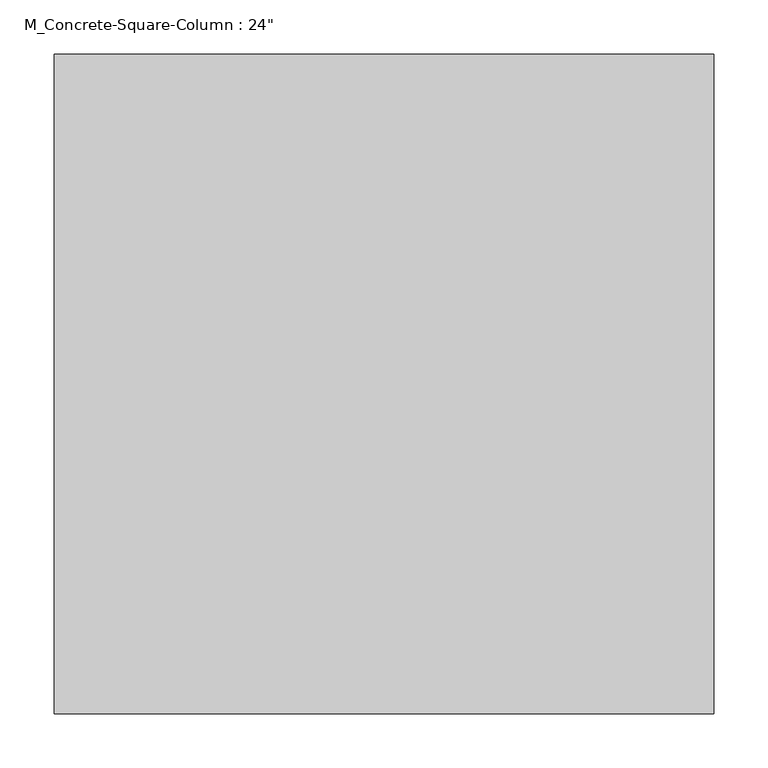
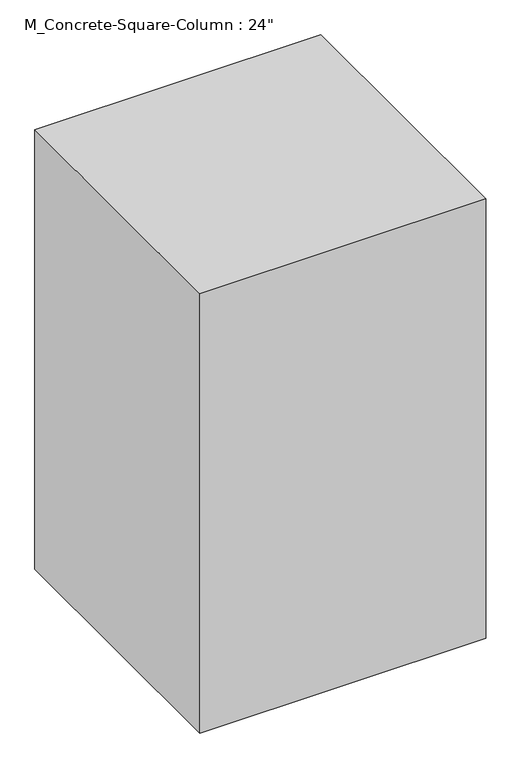
"""IFC4 building model written with IfcOpenShell, lengths in millimetres: column geometry."""

from ifc_helpers import new_model, si_unit, frame, origin, place, context, project, spatial, polyline, outline, extrude, source, transform, mapped, element, save


def column_60b89d5c(model_context):
    return source(origin(), model_context, "Body", "SweptSolid", [
        extrude(outline(polyline([(304.8, 304.8), (304.8, -304.8), (-304.8, -304.8), (-304.8, 304.8), (304.8, 304.8)])), frame((0.0, 0.0, -2133.6), z_axis=(0.0, 0.0, 1.0), x_axis=(1.0, 0.0, 0.0)), (0.0, 0.0, 1.0), 990.6),
    ])


if __name__ == "__main__":
    model = new_model("IFC4")
    model_context = context("Model", 3, world=origin())
    ifc_project = project(units=[si_unit("LENGTHUNIT", "METRE", prefix="MILLI")], contexts=[model_context])
    site = spatial("IfcSite", under=ifc_project)
    building = spatial("IfcBuilding", under=site)
    placement = place(None, origin())
    column_shape = column_60b89d5c(model_context)
    element("IfcColumn", 1, ObjectType="M_Concrete-Square-Column : 24\"", at=placement, inside=building, context=model_context, shape_type="MappedRepresentation", body=[
        mapped(column_shape, transform((0.0, 0.0, 0.0), x_axis=(1.0, 0.0, 0.0), y_axis=(0.0, 1.0, 0.0), z_axis=(0.0, 0.0, 1.0))),
    ])
    save(model, "model.ifc")

# Revit data of these elements
# Type "M_Concrete-Square-Column : 24\""
#   b = 609.6 mm
#   Structural Material [instance default] = Concrete, Cast-in-Place gray
# Element 1 (IfcColumn, "M_Concrete-Square-Column : 24\"")
#   Materials on its faces: "Concrete, Cast-in-Place gray"
# Materials
#   "Concrete, Cast-in-Place gray": class "Concrete", colour RGB 192 192 192, transparency 0, Description = "Cast-in-place concrete", Cost = 0
